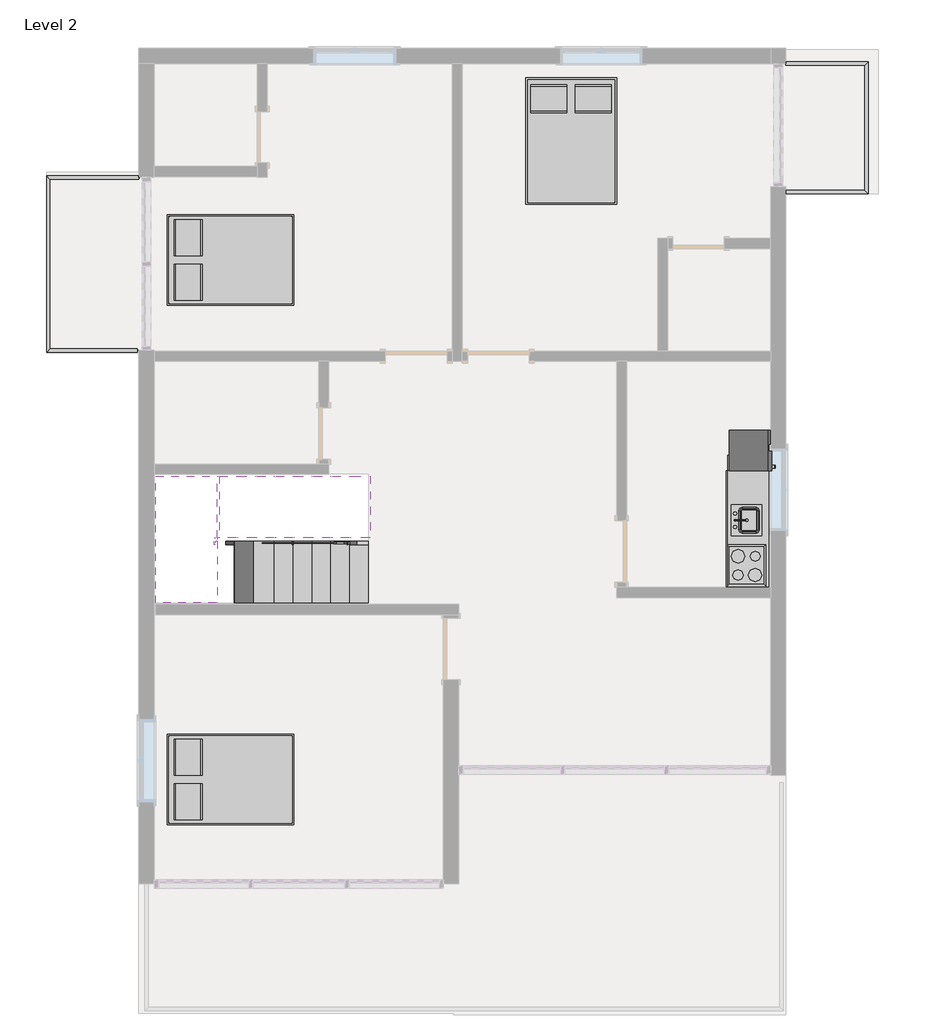
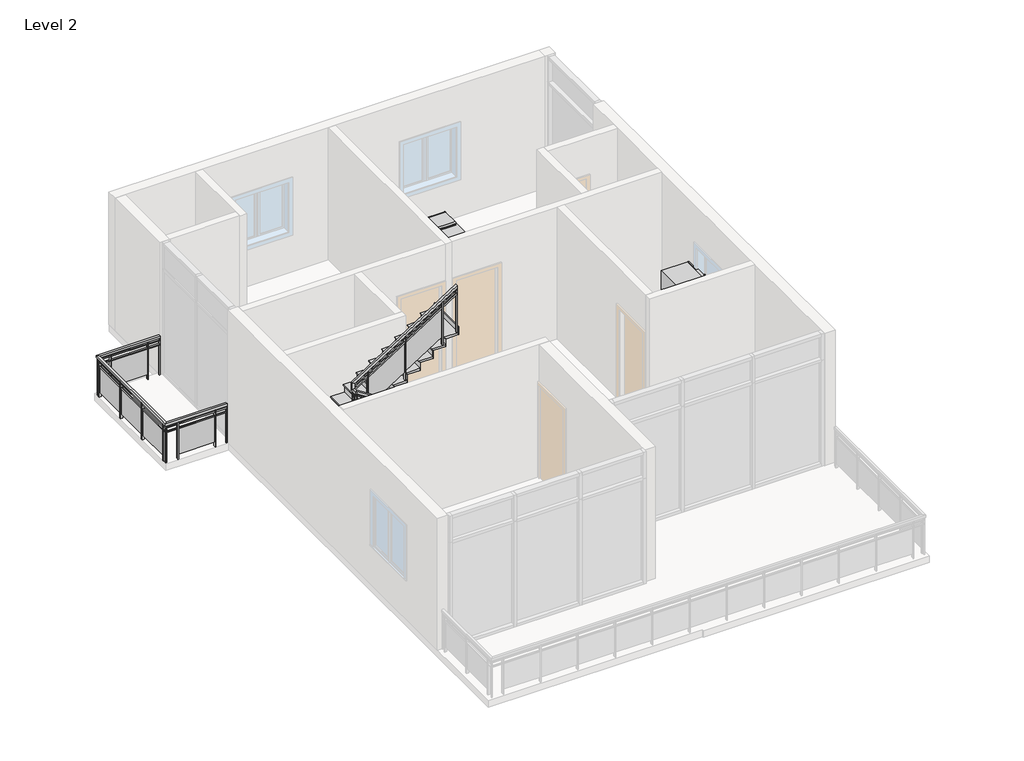
# One storey, part 3 of 3: 4 furniture elements, 4 proxies, 3 railings, 2 members, 2 stair flights, 1 flow terminal, 1 slab.
"""IFC4 building model written with IfcOpenShell, lengths in millimetres."""

from ifc_helpers import new_model, si_unit, frame, origin, place, context, project, spatial, polyline, outline, extrude, faceted_brep, transform, mapped, element, save
from components import proxy_a6faaae8, proxy_45b28599, kitchenette_medium_kitchenette_medium_844211aa, proxy_c523a7b7, flow_terminal_871c2e40, furniture_c8abb964, furniture_f14924cf, non_monolithic_landing_e910b983, stair_flight_ae0811cb, stair_flight_e53c0c70

model = new_model("IFC4")

# Units and contexts
model_context = context("Model", 3, world=origin())
ifc_project = project(units=[si_unit("LENGTHUNIT", "METRE", prefix="MILLI")], contexts=[model_context])

# Site, building, storey
site = spatial("IfcSite", under=ifc_project)
building = spatial("IfcBuilding", under=site)
storey = spatial("IfcBuildingStorey", under=building, Name="Level 2", Elevation=3200.4)

# Proxies
placement = place(None, origin())
proxy_shape = proxy_a6faaae8(model_context)
element("IfcBuildingElementProxy", 1, Name="Cook Top-4 Unit2 : 22\" x 20\"", ObjectType="Cook Top-4 Unit2 : 22\" x 20\"", at=placement, inside=storey, context=model_context, shape_type="MappedRepresentation", body=[
    mapped(proxy_shape, transform((1303.5352982, 8.7325188, 3200.4), x_axis=(0.0, 1.0000000000000002, 0.0), y_axis=(-1.0000000000000002, 0.0, 0.0), z_axis=(0.0, 0.0, 1.0))),
])
proxy_2_shape = proxy_45b28599(model_context)
element("IfcBuildingElementProxy", 2, Name="Dishwasher : 24\" x 24\" x 34\"", ObjectType="Dishwasher : 24\" x 24\" x 34\"", at=placement, inside=storey, context=model_context, shape_type="MappedRepresentation", body=[
    mapped(proxy_2_shape, transform((1595.384863, 959.9150503, 3200.4), x_axis=(0.0, 1.0000000000000002, 0.0), y_axis=(-1.0000000000000002, 0.0, 0.0), z_axis=(0.0, 0.0, 1.0))),
])
kitchenette_medium_kitchenette_medium_shape = kitchenette_medium_kitchenette_medium_844211aa(model_context)
element("IfcBuildingElementProxy", 3, Name="Kitchenette - Medium : Kitchenette - Medium", ObjectType="Kitchenette - Medium : Kitchenette - Medium", at=placement, inside=storey, context=model_context, shape_type="MappedRepresentation", body=[
    mapped(kitchenette_medium_kitchenette_medium_shape, transform((998.7352982, 332.8948139, 3200.4), x_axis=(0.0, 1.0000000000000002, 0.0), y_axis=(-1.0000000000000002, 0.0, 0.0), z_axis=(0.0, 0.0, 1.0))),
])
proxy_3_shape = proxy_c523a7b7(model_context)
element("IfcBuildingElementProxy", 4, Name="Refrigerator : 24\" x 25\" LH", ObjectType="Refrigerator : 24\" x 25\" LH", at=placement, inside=storey, context=model_context, shape_type="MappedRepresentation", body=[
    mapped(proxy_3_shape, transform((1349.1842697, 1716.8825188, 3200.4), x_axis=(0.0, 1.0000000000000002, 0.0), y_axis=(-1.0000000000000002, 0.0, 0.0), z_axis=(0.0, 0.0, 1.0))),
])

# Flow terminal
flow_terminal_shape = flow_terminal_871c2e40(model_context)
element("IfcFlowTerminal", 5, ObjectType="Sink Kitchen-Island : 18\" x 18\"", at=placement, inside=storey, context=model_context, shape_type="MappedRepresentation", body=[
    mapped(flow_terminal_shape, transform((1305.8806993, 666.1432782, 3186.0), x_axis=(0.0, 1.0000000000000002, 0.0), y_axis=(-1.0000000000000002, 0.0, 0.0), z_axis=(0.0, 0.0, 1.0))),
])

# Furniture
furniture_shape = furniture_c8abb964(model_context)
element("IfcFurniture", 6, ObjectType="Bed-Box : Double 53\" x 74\"", at=placement, inside=storey, context=model_context, shape_type="MappedRepresentation", body=[
    mapped(furniture_shape, transform((-6588.99421, 4203.4800598, 3200.4), x_axis=(0.0, 0.9999999999999999, 0.0), y_axis=(-0.9999999999999999, 0.0, 0.0), z_axis=(0.0, 0.0, 1.0))),
])
element("IfcFurniture", 7, ObjectType="Bed-Box : Double 53\" x 74\"", at=placement, inside=storey, context=model_context, shape_type="MappedRepresentation", body=[
    mapped(furniture_shape, transform((-1639.1171608, 6542.362027, 3200.4), x_axis=(1.0, 0.0, 0.0), y_axis=(0.0, 1.0, 0.0), z_axis=(0.0, 0.0, 1.0))),
])
element("IfcFurniture", 8, ObjectType="Bed-Box : Double 53\" x 74\"", at=placement, inside=storey, context=model_context, shape_type="MappedRepresentation", body=[
    mapped(furniture_shape, transform((-6588.99421, -3504.8975153, 3200.4), x_axis=(0.0, 1.0, 0.0), y_axis=(-1.0, 0.0, 0.0), z_axis=(0.0, 0.0, 1.0))),
])
furniture_2_shape = furniture_f14924cf(model_context)
element("IfcFurniture", 9, ObjectType="Counter Top w Sink Hole : 24\" Depth", at=placement, inside=storey, context=model_context, shape_type="MappedRepresentation", body=[
    mapped(furniture_2_shape, transform((998.7352982, 866.2948139, 3186.0), x_axis=(0.0, 1.0000000000000002, 0.0), y_axis=(-1.0000000000000002, 0.0, 0.0), z_axis=(0.0, 0.0, 1.0))),
])

# Members
element("IfcMember", 10, at=placement, inside=storey, context=model_context, shape_type="Brep", body=[
    faceted_brep([(-4345.5091614, 320.4049437, 3200.4), (-4543.6146908, 320.4049437, 3200.4), (-4543.6146908, 371.2049437, 3200.4), (-4345.5091614, 371.2049437, 3200.4), (-6548.9591614, 320.4049437, 4572.0), (-6548.9591614, 320.4049437, 4476.5282995), (-4345.5091614, 320.4049437, 3327.4), (-4624.9091614, 320.4049437, 3327.4), (-4624.9091614, 320.4049437, 3505.2), (-4904.3091614, 320.4049437, 3505.2), (-4904.3091614, 320.4049437, 3683.0), (-5183.7091614, 320.4049437, 3683.0), (-5183.7091614, 320.4049437, 3860.8), (-5463.1091614, 320.4049437, 3860.8), (-5463.1091614, 320.4049437, 4038.6), (-5742.5091614, 320.4049437, 4038.6), (-5742.5091614, 320.4049437, 4216.4), (-6021.9091614, 320.4049437, 4216.4), (-6021.9091614, 320.4049437, 4394.2), (-6301.3091614, 320.4049437, 4394.2), (-6301.3091614, 320.4049437, 4572.0), (-6548.9591614, 371.2049437, 4476.5282995), (-6548.9591614, 371.2049437, 4572.0), (-6301.3091614, 371.2049437, 4318.932845), (-6021.9091614, 371.2049437, 4141.132845), (-5742.5091614, 371.2049437, 3963.332845), (-5463.1091614, 371.2049437, 3785.532845), (-5183.7091614, 371.2049437, 3607.732845), (-4904.3091614, 371.2049437, 3429.932845), (-4624.9091614, 371.2049437, 3252.132845), (-4345.5091614, 371.2049437, 3327.4), (-4624.9091614, 371.2049437, 3327.4), (-4624.9091614, 371.2049437, 3505.2), (-4904.3091614, 371.2049437, 3505.2), (-4904.3091614, 371.2049437, 3683.0), (-5183.7091614, 371.2049437, 3683.0), (-5183.7091614, 371.2049437, 3860.8), (-5463.1091614, 371.2049437, 3860.8), (-5463.1091614, 371.2049437, 4038.6), (-5742.5091614, 371.2049437, 4038.6), (-5742.5091614, 371.2049437, 4216.4), (-6021.9091614, 371.2049437, 4216.4), (-6021.9091614, 371.2049437, 4394.2), (-6301.3091614, 371.2049437, 4394.2), (-6301.3091614, 371.2049437, 4572.0)], [[[0, 1, 2, 3]], [[4, 5, 1, 0, 6, 7, 8, 9, 10, 11, 12, 13, 14, 15, 16, 17, 18, 19, 20]], [[21, 5, 4, 22]], [[5, 21, 23, 24, 25, 26, 27, 28, 29, 2, 1]], [[30, 6, 0, 3]], [[6, 30, 31, 7]], [[7, 31, 32, 8]], [[8, 32, 33, 9]], [[9, 33, 34, 10]], [[10, 34, 35, 11]], [[11, 35, 36, 12]], [[12, 36, 37, 13]], [[13, 37, 38, 14]], [[14, 38, 39, 15]], [[15, 39, 40, 16]], [[16, 40, 41, 17]], [[17, 41, 42, 18]], [[18, 42, 43, 19]], [[19, 43, 44, 20]], [[20, 44, 22, 4]], [[21, 22, 44, 43, 42, 41, 40, 39, 38, 37, 36, 35, 34, 33, 32, 31, 30, 3, 2, 29, 28, 27, 26, 25, 24, 23]]]),
])
element("IfcMember", 11, at=placement, inside=storey, context=model_context, shape_type="SweptSolid", body=[
    extrude(outline(polyline([(-6599.7591614, 421.4825188), (-6548.9591614, 421.4825188), (-6548.9591614, 371.2049437), (-6580.7091614, 371.2049437), (-6580.7091614, 320.4049437), (-6599.7591614, 320.4049437), (-6599.7591614, 421.4825188)])), frame((0.0, 0.0, 4572.0), z_axis=(0.0, 0.0, 1.0), x_axis=(1.0, 0.0, 0.0)), (0.0, 0.0, 1.0), 177.8),
])

# Railings
element("IfcRailing", 12, ObjectType="Glass Panel - Bottom Fill", at=placement, inside=storey, context=model_context, shape_type="SolidModel", body=[
    faceted_brep([(-4313.7591614, 320.4049437, 4292.6), (-4313.7591614, 320.4049437, 4232.386276), (-4313.7591614, 371.2049437, 4232.386276), (-4313.7591614, 371.2049437, 4292.6), (-6548.9591614, 320.4049437, 5715.0), (-6548.9591614, 371.2049437, 5715.0), (-6548.9591614, 371.2049437, 5654.786276), (-6548.9591614, 320.4049437, 5654.786276)], [[[0, 1, 2, 3]], [[4, 5, 6, 7]], [[1, 0, 4, 7]], [[2, 1, 7, 6]], [[3, 2, 6, 5]], [[0, 3, 5, 4]]]),
    faceted_brep([(-6599.7591614, 320.4049437, 5715.0), (-6599.7591614, 320.4049437, 5664.2), (-6548.9591614, 320.4049437, 5664.2), (-6548.9591614, 320.4049437, 5715.0), (-6599.7591614, 421.4825188, 5715.0), (-6548.9591614, 421.4825188, 5715.0), (-6548.9591614, 472.2825188, 5664.2), (-6599.7591614, 472.2825188, 5664.2)], [[[0, 1, 2, 3]], [[4, 5, 6, 7]], [[1, 0, 4, 7]], [[2, 1, 7, 6]], [[3, 2, 6, 5]], [[0, 3, 5, 4]]]),
    faceted_brep([(-6599.7591614, 421.4825188, 5715.0), (-6599.7591614, 472.2825188, 5664.2), (-6548.9591614, 472.2825188, 5664.2), (-6548.9591614, 421.4825188, 5715.0), (-6599.7591614, 421.4825188, 5860.4727273), (-6548.9591614, 421.4825188, 5832.586276), (-6548.9591614, 472.2825188, 5832.586276), (-6599.7591614, 472.2825188, 5860.4727273)], [[[0, 1, 2, 3]], [[4, 5, 6, 7]], [[1, 0, 4, 7]], [[2, 1, 7, 6]], [[3, 2, 6, 5]], [[0, 3, 5, 4]]]),
    faceted_brep([(-6599.7591614, 472.2825188, 5860.4727273), (-6548.9591614, 472.2825188, 5832.586276), (-6548.9591614, 421.4825188, 5832.586276), (-6599.7591614, 421.4825188, 5860.4727273), (-4313.7591614, 472.2825188, 7315.2), (-4313.7591614, 421.4825188, 7315.2), (-4313.7591614, 421.4825188, 7254.986276), (-4313.7591614, 472.2825188, 7254.986276)], [[[0, 1, 2, 3]], [[4, 5, 6, 7]], [[1, 0, 4, 7]], [[2, 1, 7, 6]], [[3, 2, 6, 5]], [[0, 3, 5, 4]]]),
    faceted_brep([(-4313.7591614, 358.5049437, 4206.053431), (-4313.7591614, 333.1049437, 4206.053431), (-4313.7591614, 333.1049437, 4175.946569), (-4313.7591614, 358.5049437, 4175.946569), (-6545.2609127, 358.5049437, 5626.1), (-6545.2609127, 333.1049437, 5626.1), (-6552.6574102, 333.1049437, 5600.7), (-6552.6574102, 358.5049437, 5600.7), (-6561.6591614, 358.5049437, 5626.1), (-6587.0591614, 333.1049437, 5626.1), (-6587.0591614, 333.1049437, 5600.7), (-6561.6591614, 358.5049437, 5600.7), (-6561.6591614, 434.1825188, 5626.1), (-6561.6591614, 434.1825188, 5600.7), (-6587.0591614, 434.1825188, 5600.7), (-6587.0591614, 434.1825188, 5626.1)], [[[0, 1, 2, 3]], [[1, 0, 4, 5]], [[2, 1, 5, 6]], [[3, 2, 6, 7]], [[0, 3, 7, 4]], [[5, 4, 8, 9]], [[6, 5, 9, 10]], [[7, 6, 10, 11]], [[4, 7, 11, 8]], [[12, 13, 14, 15]], [[9, 8, 12, 15]], [[10, 9, 15, 14]], [[11, 10, 14, 13]], [[8, 11, 13, 12]]]),
    faceted_brep([(-6587.0591614, 434.1825188, 5782.0079765), (-6587.0591614, 459.5825188, 5782.0079765), (-6587.0591614, 459.5825188, 5751.9011144), (-6587.0591614, 434.1825188, 5751.9011144), (-4313.7591614, 434.1825188, 7228.653431), (-4313.7591614, 434.1825188, 7198.546569), (-4313.7591614, 459.5825188, 7198.546569), (-4313.7591614, 459.5825188, 7228.653431)], [[[0, 1, 2, 3]], [[4, 5, 6, 7]], [[1, 0, 4, 7]], [[2, 1, 7, 6]], [[3, 2, 6, 5]], [[0, 3, 5, 4]]]),
    faceted_brep([(-4313.7591614, 358.5049437, 4104.453431), (-4313.7591614, 333.1049437, 4104.453431), (-4313.7591614, 333.1049437, 4074.346569), (-4313.7591614, 358.5049437, 4074.346569), (-6545.2609127, 358.5049437, 5524.5), (-6545.2609127, 333.1049437, 5524.5), (-6552.6574102, 333.1049437, 5499.1), (-6552.6574102, 358.5049437, 5499.1), (-6561.6591614, 358.5049437, 5524.5), (-6587.0591614, 333.1049437, 5524.5), (-6587.0591614, 333.1049437, 5499.1), (-6561.6591614, 358.5049437, 5499.1), (-6561.6591614, 434.1825188, 5524.5), (-6561.6591614, 434.1825188, 5499.1), (-6587.0591614, 434.1825188, 5499.1), (-6587.0591614, 434.1825188, 5524.5)], [[[0, 1, 2, 3]], [[1, 0, 4, 5]], [[2, 1, 5, 6]], [[3, 2, 6, 7]], [[0, 3, 7, 4]], [[5, 4, 8, 9]], [[6, 5, 9, 10]], [[7, 6, 10, 11]], [[4, 7, 11, 8]], [[12, 13, 14, 15]], [[9, 8, 12, 15]], [[10, 9, 15, 14]], [[11, 10, 14, 13]], [[8, 11, 13, 12]]]),
    faceted_brep([(-6587.0591614, 434.1825188, 5680.4079765), (-6587.0591614, 459.5825188, 5680.4079765), (-6587.0591614, 459.5825188, 5650.3011144), (-6587.0591614, 434.1825188, 5650.3011144), (-4313.7591614, 434.1825188, 7127.053431), (-4313.7591614, 434.1825188, 7096.946569), (-4313.7591614, 459.5825188, 7096.946569), (-4313.7591614, 459.5825188, 7127.053431)], [[[0, 1, 2, 3]], [[4, 5, 6, 7]], [[1, 0, 4, 7]], [[2, 1, 7, 6]], [[3, 2, 6, 5]], [[0, 3, 5, 4]]]),
    extrude(outline(polyline([(7056.9817305, -4624.9091614), (7048.8999123, -4637.6091614), (6045.2, -4637.6091614), (6045.2, -4624.9091614), (7056.9817305, -4624.9091614)])), frame((0.0, 421.4825188, 0.0), z_axis=(0.0, 1.0, 0.0), x_axis=(0.0, 0.0, 1.0)), (0.0, 0.0, 1.0), 50.8),
    extrude(outline(polyline([(5710.3818182, -5444.0591614), (6227.6181818, -4631.2591614), (6894.9011144, -4631.2591614), (6377.6647508, -5444.0591614), (5710.3818182, -5444.0591614)])), frame((0.0, 447.0676758, 0.0), z_axis=(0.0, 1.0, 0.0), x_axis=(0.0, 0.0, 1.0)), (0.0, 0.0, 1.0), 6.35),
    extrude(outline(polyline([(6539.7453669, -5437.7091614), (6531.6635487, -5450.4091614), (5511.8, -5450.4091614), (5511.8, -5437.7091614), (6539.7453669, -5437.7091614)])), frame((0.0, 421.4825188, 0.0), z_axis=(0.0, 1.0, 0.0), x_axis=(0.0, 0.0, 1.0)), (0.0, 0.0, 1.0), 50.8),
    extrude(outline(polyline([(5176.9818182, -6256.8591614), (5694.2181818, -5444.0591614), (6377.6647508, -5444.0591614), (5860.4283872, -6256.8591614), (5176.9818182, -6256.8591614)])), frame((0.0, 447.0676758, 0.0), z_axis=(0.0, 1.0, 0.0), x_axis=(0.0, 0.0, 1.0)), (0.0, 0.0, 1.0), 6.35),
    extrude(outline(polyline([(6022.5090032, -6250.5091614), (6014.4271851, -6263.2091614), (5156.2, -6263.2091614), (5156.2, -6250.5091614), (6022.5090032, -6250.5091614)])), frame((0.0, 421.4825188, 0.0), z_axis=(0.0, 1.0, 0.0), x_axis=(0.0, 0.0, 1.0)), (0.0, 0.0, 1.0), 50.8),
    extrude(outline(polyline([(5456.7817305, -6237.8091614), (5464.8635487, -6250.5091614), (4445.0, -6250.5091614), (4445.0, -6237.8091614), (5456.7817305, -6237.8091614)])), frame((0.0, 320.4049437, 0.0), z_axis=(0.0, 1.0, 0.0), x_axis=(0.0, 0.0, 1.0)), (0.0, 0.0, 1.0), 50.8),
    extrude(outline(polyline([(4110.1818182, -5431.3591614), (4785.546569, -5431.3591614), (5302.7829326, -6244.1591614), (4627.4181818, -6244.1591614), (4110.1818182, -5431.3591614)])), frame((0.0, 339.2697867, 0.0), z_axis=(0.0, 1.0, 0.0), x_axis=(0.0, 0.0, 1.0)), (0.0, 0.0, 1.0), 6.35),
    extrude(outline(polyline([(4939.5453669, -5425.0091614), (4947.6271851, -5437.7091614), (4089.4, -5437.7091614), (4089.4, -5425.0091614), (4939.5453669, -5425.0091614)])), frame((0.0, 320.4049437, 0.0), z_axis=(0.0, 1.0, 0.0), x_axis=(0.0, 0.0, 1.0)), (0.0, 0.0, 1.0), 50.8),
    extrude(outline(polyline([(3576.7818182, -4618.5591614), (4268.3102054, -4618.5591614), (4785.546569, -5431.3591614), (4094.0181818, -5431.3591614), (3576.7818182, -4618.5591614)])), frame((0.0, 339.2697867, 0.0), z_axis=(0.0, 1.0, 0.0), x_axis=(0.0, 0.0, 1.0)), (0.0, 0.0, 1.0), 6.35),
    extrude(outline(polyline([(4422.3090032, -4612.2091614), (4430.3908214, -4624.9091614), (3556.0, -4624.9091614), (3556.0, -4612.2091614), (4422.3090032, -4612.2091614)])), frame((0.0, 320.4049437, 0.0), z_axis=(0.0, 1.0, 0.0), x_axis=(0.0, 0.0, 1.0)), (0.0, 0.0, 1.0), 50.8),
    extrude(outline(polyline([(-6583.8841614, 437.3575188), (-6583.8841614, 456.4075188), (-6564.8341614, 456.4075188), (-6564.8341614, 437.3575188), (-6583.8841614, 437.3575188)])), frame((0.0, 0.0, 4800.6), z_axis=(0.0, 0.0, 1.0), x_axis=(1.0, 0.0, 0.0)), (0.0, 0.0, 1.0), 863.6),
    extrude(outline(polyline([(5664.8885487, -6564.8341614), (5677.011276, -6583.8841614), (4800.6, -6583.8841614), (4800.6, -6564.8341614), (5664.8885487, -6564.8341614)])), frame((0.0, 336.2799437, 0.0), z_axis=(0.0, 1.0, 0.0), x_axis=(0.0, 0.0, 1.0)), (0.0, 0.0, 1.0), 19.05),
    extrude(outline(polyline([(5648.7249123, -6539.4341614), (5660.8476396, -6558.4841614), (4800.6, -6558.4841614), (4800.6, -6539.4341614), (5648.7249123, -6539.4341614)])), frame((0.0, 336.2799437, 0.0), z_axis=(0.0, 1.0, 0.0), x_axis=(0.0, 0.0, 1.0)), (0.0, 0.0, 1.0), 19.05),
    extrude(outline(polyline([(7259.0271851, -4307.4091614), (7246.9044578, -4326.4591614), (6223.0, -4326.4591614), (6223.0, -4307.4091614), (7259.0271851, -4307.4091614)])), frame((0.0, 437.3575188, 0.0), z_axis=(0.0, 1.0, 0.0), x_axis=(0.0, 0.0, 1.0)), (0.0, 0.0, 1.0), 19.05),
    extrude(outline(polyline([(4228.3453669, -4307.4091614), (4240.4680941, -4326.4591614), (3378.2, -4326.4591614), (3378.2, -4307.4091614), (4228.3453669, -4307.4091614)])), frame((0.0, 336.2799437, 0.0), z_axis=(0.0, 1.0, 0.0), x_axis=(0.0, 0.0, 1.0)), (0.0, 0.0, 1.0), 19.05),
])
element("IfcRailing", 13, ObjectType="Glass Panel - Bottom Fill", at=placement, inside=storey, context=model_context, shape_type="SolidModel", body=[
    faceted_brep([(-7713.4647018, 5742.7825188, 4114.8), (-7713.4647018, 5742.7825188, 4064.0), (-7713.4647018, 5793.5825188, 4064.0), (-7713.4647018, 5793.5825188, 4114.8), (-9034.2647018, 5742.7825188, 4114.8), (-9034.2647018, 5742.7825188, 4064.0), (-9085.0647018, 5793.5825188, 4064.0), (-9085.0647018, 5793.5825188, 4114.8), (-9034.2647018, 3228.1825188, 4114.8), (-9034.2647018, 3228.1825188, 4064.0), (-9085.0647018, 3177.3825188, 4064.0), (-9085.0647018, 3177.3825188, 4114.8), (-7738.8647018, 3228.1825188, 4114.8), (-7738.8647018, 3177.3825188, 4114.8), (-7738.8647018, 3177.3825188, 4064.0), (-7738.8647018, 3228.1825188, 4064.0)], [[[0, 1, 2, 3]], [[1, 0, 4, 5]], [[2, 1, 5, 6]], [[3, 2, 6, 7]], [[0, 3, 7, 4]], [[5, 4, 8, 9]], [[6, 5, 9, 10]], [[7, 6, 10, 11]], [[4, 7, 11, 8]], [[12, 13, 14, 15]], [[9, 8, 12, 15]], [[10, 9, 15, 14]], [[11, 10, 14, 13]], [[8, 11, 13, 12]]]),
    faceted_brep([(-7713.4647018, 5780.8825188, 4025.9), (-7713.4647018, 5755.4825188, 4025.9), (-7713.4647018, 5755.4825188, 4000.5), (-7713.4647018, 5780.8825188, 4000.5), (-9072.3647018, 5780.8825188, 4025.9), (-9046.9647018, 5755.4825188, 4025.9), (-9046.9647018, 5755.4825188, 4000.5), (-9072.3647018, 5780.8825188, 4000.5), (-9072.3647018, 3190.0825188, 4025.9), (-9046.9647018, 3215.4825188, 4025.9), (-9046.9647018, 3215.4825188, 4000.5), (-9072.3647018, 3190.0825188, 4000.5), (-7738.8647018, 3190.0825188, 4025.9), (-7738.8647018, 3190.0825188, 4000.5), (-7738.8647018, 3215.4825188, 4000.5), (-7738.8647018, 3215.4825188, 4025.9)], [[[0, 1, 2, 3]], [[1, 0, 4, 5]], [[2, 1, 5, 6]], [[3, 2, 6, 7]], [[0, 3, 7, 4]], [[5, 4, 8, 9]], [[6, 5, 9, 10]], [[7, 6, 10, 11]], [[4, 7, 11, 8]], [[12, 13, 14, 15]], [[9, 8, 12, 15]], [[10, 9, 15, 14]], [[11, 10, 14, 13]], [[8, 11, 13, 12]]]),
    faceted_brep([(-7713.4647018, 5780.8825188, 3924.3), (-7713.4647018, 5755.4825188, 3924.3), (-7713.4647018, 5755.4825188, 3898.9), (-7713.4647018, 5780.8825188, 3898.9), (-9072.3647018, 5780.8825188, 3924.3), (-9046.9647018, 5755.4825188, 3924.3), (-9046.9647018, 5755.4825188, 3898.9), (-9072.3647018, 5780.8825188, 3898.9), (-9072.3647018, 3190.0825188, 3924.3), (-9046.9647018, 3215.4825188, 3924.3), (-9046.9647018, 3215.4825188, 3898.9), (-9072.3647018, 3190.0825188, 3898.9), (-7738.8647018, 3190.0825188, 3924.3), (-7738.8647018, 3190.0825188, 3898.9), (-7738.8647018, 3215.4825188, 3898.9), (-7738.8647018, 3215.4825188, 3924.3)], [[[0, 1, 2, 3]], [[1, 0, 4, 5]], [[2, 1, 5, 6]], [[3, 2, 6, 7]], [[0, 3, 7, 4]], [[5, 4, 8, 9]], [[6, 5, 9, 10]], [[7, 6, 10, 11]], [[4, 7, 11, 8]], [[12, 13, 14, 15]], [[9, 8, 12, 15]], [[10, 9, 15, 14]], [[11, 10, 14, 13]], [[8, 11, 13, 12]]]),
    extrude(outline(polyline([(-7999.2147018, 3177.3825188), (-7999.2147018, 3228.1825188), (-7986.5147018, 3228.1825188), (-7986.5147018, 3177.3825188), (-7999.2147018, 3177.3825188)])), frame((0.0, 0.0, 3200.4), z_axis=(0.0, 0.0, 1.0), x_axis=(1.0, 0.0, 0.0)), (0.0, 0.0, 1.0), 863.6),
    extrude(outline(polyline([(-8805.6647018, 3209.3176758), (-7992.8647018, 3209.3176758), (-7992.8647018, 3202.9676758), (-8805.6647018, 3202.9676758), (-8805.6647018, 3209.3176758)])), frame((0.0, 0.0, 3302.0), z_axis=(0.0, 0.0, 1.0), x_axis=(1.0, 0.0, 0.0)), (0.0, 0.0, 1.0), 596.9),
    extrude(outline(polyline([(-8812.0147018, 3177.3825188), (-8812.0147018, 3228.1825188), (-8799.3147018, 3228.1825188), (-8799.3147018, 3177.3825188), (-8812.0147018, 3177.3825188)])), frame((0.0, 0.0, 3200.4), z_axis=(0.0, 0.0, 1.0), x_axis=(1.0, 0.0, 0.0)), (0.0, 0.0, 1.0), 863.6),
    extrude(outline(polyline([(-9085.0647018, 3272.6325188), (-9034.2647018, 3272.6325188), (-9034.2647018, 3259.9325188), (-9085.0647018, 3259.9325188), (-9085.0647018, 3272.6325188)])), frame((0.0, 0.0, 3200.4), z_axis=(0.0, 0.0, 1.0), x_axis=(1.0, 0.0, 0.0)), (0.0, 0.0, 1.0), 863.6),
    extrude(outline(polyline([(-9053.1295448, 4079.0825188), (-9053.1295448, 3266.2825188), (-9059.4795448, 3266.2825188), (-9059.4795448, 4079.0825188), (-9053.1295448, 4079.0825188)])), frame((0.0, 0.0, 3302.0), z_axis=(0.0, 0.0, 1.0), x_axis=(1.0, 0.0, 0.0)), (0.0, 0.0, 1.0), 596.9),
    extrude(outline(polyline([(-9085.0647018, 4085.4325188), (-9034.2647018, 4085.4325188), (-9034.2647018, 4072.7325188), (-9085.0647018, 4072.7325188), (-9085.0647018, 4085.4325188)])), frame((0.0, 0.0, 3200.4), z_axis=(0.0, 0.0, 1.0), x_axis=(1.0, 0.0, 0.0)), (0.0, 0.0, 1.0), 863.6),
    extrude(outline(polyline([(-9053.1295448, 4891.8825188), (-9053.1295448, 4079.0825188), (-9059.4795448, 4079.0825188), (-9059.4795448, 4891.8825188), (-9053.1295448, 4891.8825188)])), frame((0.0, 0.0, 3302.0), z_axis=(0.0, 0.0, 1.0), x_axis=(1.0, 0.0, 0.0)), (0.0, 0.0, 1.0), 596.9),
    extrude(outline(polyline([(-9085.0647018, 4898.2325188), (-9034.2647018, 4898.2325188), (-9034.2647018, 4885.5325188), (-9085.0647018, 4885.5325188), (-9085.0647018, 4898.2325188)])), frame((0.0, 0.0, 3200.4), z_axis=(0.0, 0.0, 1.0), x_axis=(1.0, 0.0, 0.0)), (0.0, 0.0, 1.0), 863.6),
    extrude(outline(polyline([(-9053.1295448, 5704.6825188), (-9053.1295448, 4891.8825188), (-9059.4795448, 4891.8825188), (-9059.4795448, 5704.6825188), (-9053.1295448, 5704.6825188)])), frame((0.0, 0.0, 3302.0), z_axis=(0.0, 0.0, 1.0), x_axis=(1.0, 0.0, 0.0)), (0.0, 0.0, 1.0), 596.9),
    extrude(outline(polyline([(-9085.0647018, 5711.0325188), (-9034.2647018, 5711.0325188), (-9034.2647018, 5698.3325188), (-9085.0647018, 5698.3325188), (-9085.0647018, 5711.0325188)])), frame((0.0, 0.0, 3200.4), z_axis=(0.0, 0.0, 1.0), x_axis=(1.0, 0.0, 0.0)), (0.0, 0.0, 1.0), 863.6),
    extrude(outline(polyline([(-8786.6147018, 5793.5825188), (-8786.6147018, 5742.7825188), (-8799.3147018, 5742.7825188), (-8799.3147018, 5793.5825188), (-8786.6147018, 5793.5825188)])), frame((0.0, 0.0, 3200.4), z_axis=(0.0, 0.0, 1.0), x_axis=(1.0, 0.0, 0.0)), (0.0, 0.0, 1.0), 863.6),
    extrude(outline(polyline([(-7980.1647018, 5761.6473618), (-8792.9647018, 5761.6473618), (-8792.9647018, 5767.9973618), (-7980.1647018, 5767.9973618), (-7980.1647018, 5761.6473618)])), frame((0.0, 0.0, 3302.0), z_axis=(0.0, 0.0, 1.0), x_axis=(1.0, 0.0, 0.0)), (0.0, 0.0, 1.0), 596.9),
    extrude(outline(polyline([(-7973.8147018, 5793.5825188), (-7973.8147018, 5742.7825188), (-7986.5147018, 5742.7825188), (-7986.5147018, 5793.5825188), (-7973.8147018, 5793.5825188)])), frame((0.0, 0.0, 3200.4), z_axis=(0.0, 0.0, 1.0), x_axis=(1.0, 0.0, 0.0)), (0.0, 0.0, 1.0), 863.6),
    extrude(outline(polyline([(-9069.1897018, 3212.3075188), (-9050.1397018, 3212.3075188), (-9050.1397018, 3193.2575188), (-9069.1897018, 3193.2575188), (-9069.1897018, 3212.3075188)])), frame((0.0, 0.0, 3200.4), z_axis=(0.0, 0.0, 1.0), x_axis=(1.0, 0.0, 0.0)), (0.0, 0.0, 1.0), 863.6),
    extrude(outline(polyline([(-9050.1397018, 5777.7075188), (-9050.1397018, 5758.6575188), (-9069.1897018, 5758.6575188), (-9069.1897018, 5777.7075188), (-9050.1397018, 5777.7075188)])), frame((0.0, 0.0, 3200.4), z_axis=(0.0, 0.0, 1.0), x_axis=(1.0, 0.0, 0.0)), (0.0, 0.0, 1.0), 863.6),
    extrude(outline(polyline([(-7751.5647018, 3193.2575188), (-7751.5647018, 3212.3075188), (-7732.5147018, 3212.3075188), (-7732.5147018, 3193.2575188), (-7751.5647018, 3193.2575188)])), frame((0.0, 0.0, 3200.4), z_axis=(0.0, 0.0, 1.0), x_axis=(1.0, 0.0, 0.0)), (0.0, 0.0, 1.0), 863.6),
    extrude(outline(polyline([(-7707.1147018, 5777.7075188), (-7707.1147018, 5758.6575188), (-7726.1647018, 5758.6575188), (-7726.1647018, 5777.7075188), (-7707.1147018, 5777.7075188)])), frame((0.0, 0.0, 3200.4), z_axis=(0.0, 0.0, 1.0), x_axis=(1.0, 0.0, 0.0)), (0.0, 0.0, 1.0), 863.6),
])
element("IfcRailing", 14, ObjectType="Glass Panel - Bottom Fill", at=placement, inside=storey, context=model_context, shape_type="SolidModel", body=[
    faceted_brep([(1887.7352982, 7482.6825188, 4114.8), (1887.7352982, 7482.6825188, 4064.0), (1887.7352982, 7431.8825188, 4064.0), (1887.7352982, 7431.8825188, 4114.8), (3106.9352982, 7482.6825188, 4114.8), (3106.9352982, 7482.6825188, 4064.0), (3056.1352982, 7431.8825188, 4064.0), (3056.1352982, 7431.8825188, 4114.8), (3106.9352982, 5526.8825188, 4114.8), (3106.9352982, 5526.8825188, 4064.0), (3056.1352982, 5577.6825188, 4064.0), (3056.1352982, 5577.6825188, 4114.8), (1887.7352982, 5526.8825188, 4114.8), (1887.7352982, 5577.6825188, 4114.8), (1887.7352982, 5577.6825188, 4064.0), (1887.7352982, 5526.8825188, 4064.0)], [[[0, 1, 2, 3]], [[1, 0, 4, 5]], [[2, 1, 5, 6]], [[3, 2, 6, 7]], [[0, 3, 7, 4]], [[5, 4, 8, 9]], [[6, 5, 9, 10]], [[7, 6, 10, 11]], [[4, 7, 11, 8]], [[12, 13, 14, 15]], [[9, 8, 12, 15]], [[10, 9, 15, 14]], [[11, 10, 14, 13]], [[8, 11, 13, 12]]]),
    faceted_brep([(1887.7352982, 7444.5825188, 4025.9), (1887.7352982, 7469.9825188, 4025.9), (1887.7352982, 7469.9825188, 4000.5), (1887.7352982, 7444.5825188, 4000.5), (3068.8352982, 7444.5825188, 4025.9), (3094.2352982, 7469.9825188, 4025.9), (3094.2352982, 7469.9825188, 4000.5), (3068.8352982, 7444.5825188, 4000.5), (3068.8352982, 5564.9825188, 4025.9), (3094.2352982, 5539.5825188, 4025.9), (3094.2352982, 5539.5825188, 4000.5), (3068.8352982, 5564.9825188, 4000.5), (1887.7352982, 5564.9825188, 4025.9), (1887.7352982, 5564.9825188, 4000.5), (1887.7352982, 5539.5825188, 4000.5), (1887.7352982, 5539.5825188, 4025.9)], [[[0, 1, 2, 3]], [[1, 0, 4, 5]], [[2, 1, 5, 6]], [[3, 2, 6, 7]], [[0, 3, 7, 4]], [[5, 4, 8, 9]], [[6, 5, 9, 10]], [[7, 6, 10, 11]], [[4, 7, 11, 8]], [[12, 13, 14, 15]], [[9, 8, 12, 15]], [[10, 9, 15, 14]], [[11, 10, 14, 13]], [[8, 11, 13, 12]]]),
    faceted_brep([(1887.7352982, 7444.5825188, 3924.3), (1887.7352982, 7469.9825188, 3924.3), (1887.7352982, 7469.9825188, 3898.9), (1887.7352982, 7444.5825188, 3898.9), (3068.8352982, 7444.5825188, 3924.3), (3094.2352982, 7469.9825188, 3924.3), (3094.2352982, 7469.9825188, 3898.9), (3068.8352982, 7444.5825188, 3898.9), (3068.8352982, 5564.9825188, 3924.3), (3094.2352982, 5539.5825188, 3924.3), (3094.2352982, 5539.5825188, 3898.9), (3068.8352982, 5564.9825188, 3898.9), (1887.7352982, 5564.9825188, 3924.3), (1887.7352982, 5564.9825188, 3898.9), (1887.7352982, 5539.5825188, 3898.9), (1887.7352982, 5539.5825188, 3924.3)], [[[0, 1, 2, 3]], [[1, 0, 4, 5]], [[2, 1, 5, 6]], [[3, 2, 6, 7]], [[0, 3, 7, 4]], [[5, 4, 8, 9]], [[6, 5, 9, 10]], [[7, 6, 10, 11]], [[4, 7, 11, 8]], [[12, 13, 14, 15]], [[9, 8, 12, 15]], [[10, 9, 15, 14]], [[11, 10, 14, 13]], [[8, 11, 13, 12]]]),
    extrude(outline(polyline([(2084.5852982, 5577.6825188), (2084.5852982, 5526.8825188), (2071.8852982, 5526.8825188), (2071.8852982, 5577.6825188), (2084.5852982, 5577.6825188)])), frame((0.0, 0.0, 3200.4), z_axis=(0.0, 0.0, 1.0), x_axis=(1.0, 0.0, 0.0)), (0.0, 0.0, 1.0), 863.6),
    extrude(outline(polyline([(2891.0352982, 5545.7473618), (2078.2352982, 5545.7473618), (2078.2352982, 5552.0973618), (2891.0352982, 5552.0973618), (2891.0352982, 5545.7473618)])), frame((0.0, 0.0, 3302.0), z_axis=(0.0, 0.0, 1.0), x_axis=(1.0, 0.0, 0.0)), (0.0, 0.0, 1.0), 596.9),
    extrude(outline(polyline([(2897.3852982, 5577.6825188), (2897.3852982, 5526.8825188), (2884.6852982, 5526.8825188), (2884.6852982, 5577.6825188), (2897.3852982, 5577.6825188)])), frame((0.0, 0.0, 3200.4), z_axis=(0.0, 0.0, 1.0), x_axis=(1.0, 0.0, 0.0)), (0.0, 0.0, 1.0), 863.6),
    extrude(outline(polyline([(3056.1352982, 5698.3325188), (3106.9352982, 5698.3325188), (3106.9352982, 5685.6325188), (3056.1352982, 5685.6325188), (3056.1352982, 5698.3325188)])), frame((0.0, 0.0, 3200.4), z_axis=(0.0, 0.0, 1.0), x_axis=(1.0, 0.0, 0.0)), (0.0, 0.0, 1.0), 863.6),
    extrude(outline(polyline([(3088.0704552, 6504.7825188), (3088.0704552, 5691.9825188), (3081.7204552, 5691.9825188), (3081.7204552, 6504.7825188), (3088.0704552, 6504.7825188)])), frame((0.0, 0.0, 3302.0), z_axis=(0.0, 0.0, 1.0), x_axis=(1.0, 0.0, 0.0)), (0.0, 0.0, 1.0), 596.9),
    extrude(outline(polyline([(3056.1352982, 6511.1325188), (3106.9352982, 6511.1325188), (3106.9352982, 6498.4325188), (3056.1352982, 6498.4325188), (3056.1352982, 6511.1325188)])), frame((0.0, 0.0, 3200.4), z_axis=(0.0, 0.0, 1.0), x_axis=(1.0, 0.0, 0.0)), (0.0, 0.0, 1.0), 863.6),
    extrude(outline(polyline([(3088.0704552, 7317.5825188), (3088.0704552, 6504.7825188), (3081.7204552, 6504.7825188), (3081.7204552, 7317.5825188), (3088.0704552, 7317.5825188)])), frame((0.0, 0.0, 3302.0), z_axis=(0.0, 0.0, 1.0), x_axis=(1.0, 0.0, 0.0)), (0.0, 0.0, 1.0), 596.9),
    extrude(outline(polyline([(3056.1352982, 7323.9325188), (3106.9352982, 7323.9325188), (3106.9352982, 7311.2325188), (3056.1352982, 7311.2325188), (3056.1352982, 7323.9325188)])), frame((0.0, 0.0, 3200.4), z_axis=(0.0, 0.0, 1.0), x_axis=(1.0, 0.0, 0.0)), (0.0, 0.0, 1.0), 863.6),
    extrude(outline(polyline([(2884.6852982, 7431.8825188), (2884.6852982, 7482.6825188), (2897.3852982, 7482.6825188), (2897.3852982, 7431.8825188), (2884.6852982, 7431.8825188)])), frame((0.0, 0.0, 3200.4), z_axis=(0.0, 0.0, 1.0), x_axis=(1.0, 0.0, 0.0)), (0.0, 0.0, 1.0), 863.6),
    extrude(outline(polyline([(2078.2352982, 7463.8176758), (2891.0352982, 7463.8176758), (2891.0352982, 7457.4676758), (2078.2352982, 7457.4676758), (2078.2352982, 7463.8176758)])), frame((0.0, 0.0, 3302.0), z_axis=(0.0, 0.0, 1.0), x_axis=(1.0, 0.0, 0.0)), (0.0, 0.0, 1.0), 596.9),
    extrude(outline(polyline([(2071.8852982, 7431.8825188), (2071.8852982, 7482.6825188), (2084.5852982, 7482.6825188), (2084.5852982, 7431.8825188), (2071.8852982, 7431.8825188)])), frame((0.0, 0.0, 3200.4), z_axis=(0.0, 0.0, 1.0), x_axis=(1.0, 0.0, 0.0)), (0.0, 0.0, 1.0), 863.6),
    extrude(outline(polyline([(3072.0102982, 5561.8075188), (3091.0602982, 5561.8075188), (3091.0602982, 5542.7575188), (3072.0102982, 5542.7575188), (3072.0102982, 5561.8075188)])), frame((0.0, 0.0, 3200.4), z_axis=(0.0, 0.0, 1.0), x_axis=(1.0, 0.0, 0.0)), (0.0, 0.0, 1.0), 863.6),
    extrude(outline(polyline([(3072.0102982, 7447.7575188), (3072.0102982, 7466.8075188), (3091.0602982, 7466.8075188), (3091.0602982, 7447.7575188), (3072.0102982, 7447.7575188)])), frame((0.0, 0.0, 3200.4), z_axis=(0.0, 0.0, 1.0), x_axis=(1.0, 0.0, 0.0)), (0.0, 0.0, 1.0), 863.6),
    extrude(outline(polyline([(1900.4352982, 5561.8075188), (1900.4352982, 5542.7575188), (1881.3852982, 5542.7575188), (1881.3852982, 5561.8075188), (1900.4352982, 5561.8075188)])), frame((0.0, 0.0, 3200.4), z_axis=(0.0, 0.0, 1.0), x_axis=(1.0, 0.0, 0.0)), (0.0, 0.0, 1.0), 863.6),
    extrude(outline(polyline([(1881.3852982, 7447.7575188), (1881.3852982, 7466.8075188), (1900.4352982, 7466.8075188), (1900.4352982, 7447.7575188), (1881.3852982, 7447.7575188)])), frame((0.0, 0.0, 3200.4), z_axis=(0.0, 0.0, 1.0), x_axis=(1.0, 0.0, 0.0)), (0.0, 0.0, 1.0), 863.6),
])

# Slab
non_monolithic_landing_shape = non_monolithic_landing_e910b983(model_context)
element("IfcSlab", 15, ObjectType="Non-Monolithic Landing", at=placement, inside=storey, context=model_context, shape_type="MappedRepresentation", body=[
    mapped(non_monolithic_landing_shape, transform((0.0, 0.0, 0.0), x_axis=(1.0, 0.0, 0.0), y_axis=(0.0, 1.0, 0.0), z_axis=(0.0, 0.0, 1.0))),
])

# Stair flights
stair_flight_shape = stair_flight_ae0811cb(model_context)
element("IfcStairFlight", 16, ObjectType="2\" Tread 1\" Nosing 1/4\" Riser", at=placement, inside=storey, context=model_context, shape_type="MappedRepresentation", body=[
    mapped(stair_flight_shape, transform((0.0, 0.0, 0.0), x_axis=(1.0, 0.0, 0.0), y_axis=(0.0, 1.0, 0.0), z_axis=(0.0, 0.0, 1.0))),
])
stair_flight_2_shape = stair_flight_e53c0c70(model_context)
element("IfcStairFlight", 17, ObjectType="2\" Tread 1\" Nosing 1/4\" Riser", at=placement, inside=storey, context=model_context, shape_type="MappedRepresentation", body=[
    mapped(stair_flight_2_shape, transform((0.0, 0.0, 0.0), x_axis=(1.0, 0.0, 0.0), y_axis=(0.0, 1.0, 0.0), z_axis=(0.0, 0.0, 1.0))),
])

save(model, "model.ifc")

# Revit data of these elements
# Type "Cook Top-4 Unit2 : 22\" x 20\""
#   Depth = 1' - 8"
#   Width = 1' - 10"
#   Burner Material = Steel, Chrome Plated
#   Cooktop Material = Steel, Polished
#   Default Elevation = 0
#   Assembly Code = ""
# Type "Dishwasher : 24\" x 24\" x 34\""
#   Label = "DW"
#   Assembly Code = "E1090400"
#   Depth = 2' - 0"
#   Height = 2' - 10"
#   Width = 2' - 0"
#   Dishwasher Material = Steel, Paint Finish, Ivory, Glossy
#   Panel Face Material = Plastic, Opaque Black
#   Default Elevation = 0
# Type "Kitchenette - Medium : Kitchenette - Medium"
#   Assembly Code = "E1090400"
#   Counter Length = 5' - 9"
#   Cabinet Width = 4' - 6"
#   Cabinet Height = 2' - 10 1/2"
#   Cabinet Depth = 2' - 0"
#   Toe Depth = 0' - 3"
#   Toe Height = 0' - 3 1/2"
#   Cabinet Material = Cabinets
#   Door/Drawer Material = Cabinets
#   Handle Material = Cabinets - Handles
#   Default Elevation = 0
# Type "Refrigerator : 24\" x 25\" LH"
#   Label = "REF."
#   Assembly Code = "E1090400"
#   Depth = 2' - 0 3/4"
#   Handle = 0' - 1 1/2"
#   Height = 5' - 3 1/2"
#   Rear Clearance = 0' - 2"
#   Top Door Height = 1' - 8"
#   Width = 1' - 11 1/2"
#   Material = Steel, Paint Finish, Ivory, Glossy
#   Default Elevation = 0
# Type "Sink Kitchen-Island : 18\" x 18\""
#   Assembly Code = "D2010410"
#   Counter Height = 3' - 0"
#   Depth = 1' - 6"
#   Width = 1' - 6"
#   Faucet Material = Steel, Polished
#   Sink Material = Steel, Polished
#   Default Elevation = 0
# Type "Bed-Box : Double 53\" x 74\""
#   Assembly Code = "E2020200"
#   Length = 6' - 2"
#   Width = 4' - 5"
#   Frame Material = Birch
#   Mattress Material = Linen, White
#   Default Elevation = 0
# Type "Counter Top w Sink Hole : 24\" Depth"
#   Assembly Code = "C1030400"
#   Counter Thickness = 0' - 1 1/2"
#   Depth = 2' - 1"
#   Height = 3' - 0"
#   Length [instance default] = 8' - 0"
#   Sink Location [instance default] = 2' - 0"
#   Sink Location To Wall [instance default] = 0' - 6"
#   Sink Opening Depth [instance default] = 1' - 3"
#   Sink Opening Width [instance default] = 2' - 3"
#   Counter Top Material = none
#   Default Elevation = 0
# Type "Glass Panel - Bottom Fill"
#   Assembly Code = "C2010400"
#   built-in parameter 1008612 = 0.0416667 (stored number, unit not read)
#   built-in parameter 1008611 = 0.0416667 (stored number, unit not read)
#   built-in parameter 1008609 = 0.333333 (stored number, unit not read)
#   built-in parameter 1008604 = 0.166667 (stored number, unit not read)
#   built-in parameter 1008603 = 0.166667 (stored number, unit not read)
#   Railing Height = 3' - 0"
#   built-in parameter 1008630 = 2
#   built-in parameter 1008610 = 2
#   built-in parameter 1008618 = Baluster - Square : 3/4"
# Element 1 (IfcBuildingElementProxy, "Cook Top-4 Unit2 : 22\" x 20\"")
#   Phase Created = New Construction
#   Materials on its faces: "Steel, Chrome Plated", "Steel, Polished"
# Element 2 (IfcBuildingElementProxy, "Dishwasher : 24\" x 24\" x 34\"")
#   Phase Created = New Construction
#   Materials on its faces: "Steel, Paint Finish, Ivory, Glossy", "Plastic, Opaque Black"
# Element 3 (IfcBuildingElementProxy, "Kitchenette - Medium : Kitchenette - Medium")
#   Phase Created = New Construction
#   Materials on its faces: "Cabinets", "Cabinets - Handles"
# Element 4 (IfcBuildingElementProxy, "Refrigerator : 24\" x 25\" LH")
#   Phase Created = New Construction
#   Materials on its faces: "Steel, Paint Finish, Ivory, Glossy", "Steel, Chrome Plated"
# Element 5 (IfcFlowTerminal, "Sink Kitchen-Island : 18\" x 18\"")
#   Mark = "8"
#   Phase Created = New Construction
#   Materials on its faces: "Steel, Polished"
# Elements 6, 7, 8 (IfcFurniture, "Bed-Box : Double 53\" x 74\"")
#   Phase Created = New Construction
#   Materials on its faces: "Birch", "Linen, White"
# Element 9 (IfcFurniture, "Counter Top w Sink Hole : 24\" Depth")
#   Sink Opening Depth = 1' - 2"
#   Sink Location To Wall = 0' - 6"
#   Length = 5' - 9"
#   Sink Location = 3' - 4"
#   Sink Opening Width = 1' - 4"
#   Phase Created = New Construction
#   Materials on its faces: "Counter Top"
# Elements 10, 11 (IfcMember)
#   Phase Created = New Construction
# Elements 12, 13, 14 (IfcRailing, "Glass Panel - Bottom Fill")
#   Phase Created = New Construction
#   Materials on its faces: "Glass"
# Element 15 (IfcSlab, "Non-Monolithic Landing")
#   Phase Created = New Construction
# Elements 16, 17 (IfcStairFlight, "2\" Tread 1\" Nosing 1/4\" Riser")
#   Phase Created = New Construction
# Materials
#   "Steel, Chrome Plated": class "Metal", colour RGB 17 17 17, transparency 0, Description = "Chromiuim plated steel", Cost = 0
#   "Steel, Polished": class "Metal", colour RGB 57 57 57, transparency 0, Description = "Polished steel", Cost = 0
#   "Steel, Paint Finish, Ivory, Glossy": class "Metal", colour RGB 247 247 239, transparency 0, Description = "Steel, paint finish, ivory, glossy", Cost = 0
#   "Plastic, Opaque Black": class "Plastic", colour RGB 0 0 0, transparency 0.7, Description = "Plastic, generic, opaque black", Cost = 0
#   "Cabinets": colour RGB 249 249 249, transparency 0
#   "Cabinets - Handles": class "Metal", colour RGB 57 57 57, transparency 0
#   "Birch": class "Wood", colour RGB 224 178 126, transparency 0, Description = "Betula Alleghaniensis", Cost = 0
#   "Linen, White": class "Textile", colour RGB 247 247 239, transparency 0, Description = "Linen, white", Cost = 0
#   "Counter Top": class "Wood", colour RGB 226 177 128, transparency 0
#   "Glass": class "Glass", colour RGB 0 128 192, transparency 0.75, Description = "Soda Lime Glass", Cost = 0
